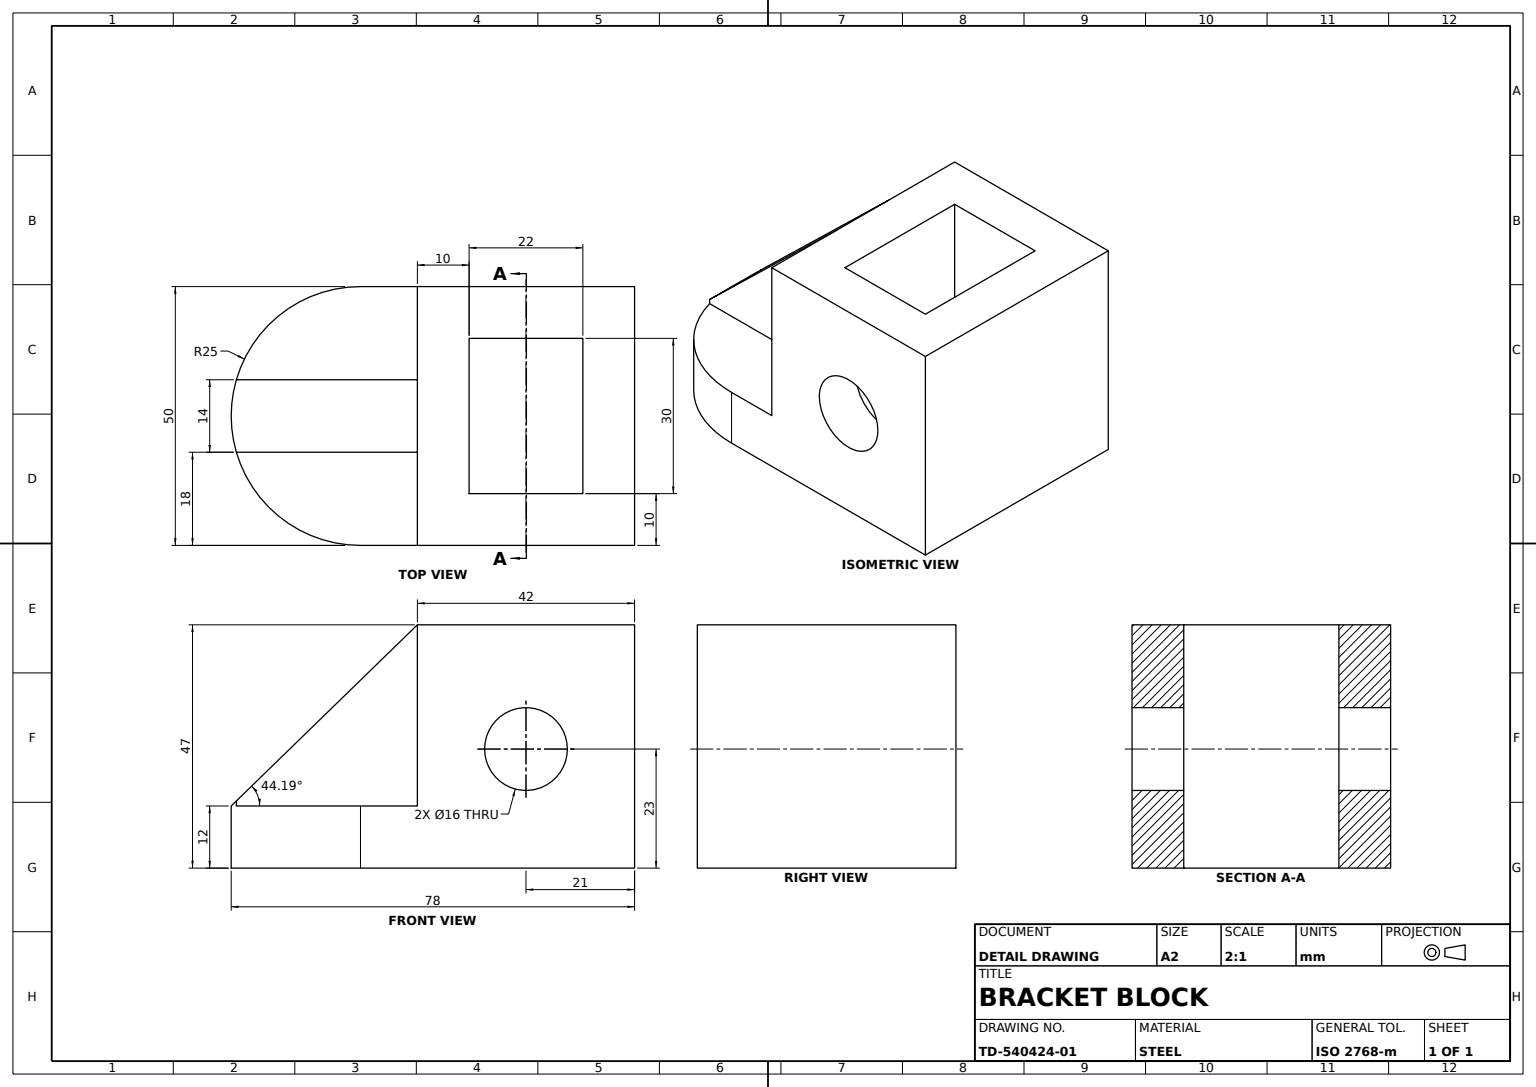
from build123d import *

# Parameters (mm, degrees)
BASE_PLATE_SKETCH_W      = 78
BASE_PLATE_SKETCH_H      = 12
BASE_PLATE_DEPTH         = 50
UPRIGHT_BLOCK_SKETCH_W   = 42
UPRIGHT_BLOCK_SKETCH_H   = 35
UPRIGHT_BLOCK_DEPTH      = 50
BLOCK_POCKET_SKETCH_W    = 30
BLOCK_POCKET_SKETCH_H    = 22
BLOCK_POCKET_30X22_DEPTH = 79.930349043
SIDE_CUT_1_SKETCH_R      = 8
SIDE_CUT_1_DEPTH         = 10
SIDE_START               = -10
SIDE_CUT_2_SKETCH_R      = 8
SIDE_CUT_2_DEPTH         = 10
GUSSET_RIB_14MM_REACH    = 63.863
GUSSET_RIB_SKETCH_WALL_W = 175.935063468
GUSSET_RIB_SKETCH_WALL_H = 14
FRONT_PROFILE_CUT_DEPTH  = 73.429275849
RIB_START                = -20
RIB_TRIM_CUT_DEPTH       = 20


with BuildPart() as part:
    # Base Plate Sketch → Base Plate (new body)
    with BuildSketch(Plane(origin=(0, 0, 0), x_dir=(0, 0, -1), z_dir=(1, 0, 0))):
        Rectangle(BASE_PLATE_SKETCH_W, BASE_PLATE_SKETCH_H)
    extrude(amount=-BASE_PLATE_DEPTH)

    # Upright Block Sketch → Upright Block (add)
    with BuildSketch(Plane(origin=(0, 0, 0), x_dir=(0, 0, -1), z_dir=(1, 0, 0))):
        with Locations((18, 23.5)):
            Rectangle(UPRIGHT_BLOCK_SKETCH_W, UPRIGHT_BLOCK_SKETCH_H)
    extrude(amount=-UPRIGHT_BLOCK_DEPTH)

    # Block Pocket Sketch → Block Pocket 30x22 (cut, through all)
    with BuildSketch(Plane(origin=(0, 41, 0), x_dir=(1, 0, 0), z_dir=(0, 1, 0))):
        with Locations((-25, 18)):
            Rectangle(BLOCK_POCKET_SKETCH_W, BLOCK_POCKET_SKETCH_H)
    extrude(amount=-BLOCK_POCKET_30X22_DEPTH, mode=Mode.SUBTRACT)

    # Side Cut 1 Sketch → Side Cut 1 (cut)
    with BuildSketch(Plane(origin=(0, 0, 0), x_dir=(0, 0, -1), z_dir=(1, 0, 0))):
        with Locations((18, 17)):
            Circle(SIDE_CUT_1_SKETCH_R)
    extrude(amount=-SIDE_CUT_1_DEPTH, mode=Mode.SUBTRACT)

    # Side Cut 2 Sketch → Side Cut 2 (cut)
    with BuildSketch(Plane.ZY.offset(50).offset(SIDE_START)):
        with Locations(Location((-18, 17, 0), (0, 0, 180))):
            Circle(SIDE_CUT_2_SKETCH_R)
    extrude(amount=SIDE_CUT_2_DEPTH, mode=Mode.SUBTRACT)

    # Gusset Rib Sketch wall → Gusset Rib 14mm (add, up to next)
    with BuildSketch(Plane(origin=(-25, 23.5, 21), x_dir=(0, 0.697078393292, -0.716994918814), z_dir=(0, 0.716994918814, 0.697078393292)), mode=Mode.PRIVATE) as gusset_rib_14mm_sk1:
        Rectangle(GUSSET_RIB_SKETCH_WALL_W, GUSSET_RIB_SKETCH_WALL_H)
    gusset_rib_14mm_tool1 = extrude(gusset_rib_14mm_sk1.sketch, amount=-GUSSET_RIB_14MM_REACH, mode=Mode.PRIVATE) - part.part
    add(gusset_rib_14mm_tool1.solids().sort_by_distance((-25, 23.5, 21))[0])

    # Front Profile Cut Sketch → Front Profile Cut (cut, through all)
    with BuildSketch(Plane(origin=(0, 6, 0), x_dir=(1, 0, 0), z_dir=(0, 1, 0))):
        with BuildLine():
            Line((-50, -39), (-25, -39))
            ThreePointArc((-25, -39), (-42.67766953, -31.67766953), (-50, -14))
            Line((-50, -14), (-50, -39))
        make_face()
        with BuildLine():
            Line((-18, -38), (-18, -39))
            Line((-18, -39), (0, -39))
            Line((0, -39), (0, -14))
            ThreePointArc((0, -14), (-5, -29), (-18, -38))
        make_face()
    extrude(amount=-FRONT_PROFILE_CUT_DEPTH, mode=Mode.SUBTRACT)

    # Rib Trim Cut Sketch → Rib Trim Cut (cut)
    with BuildSketch(Plane.XZ.offset(6).offset(RIB_START)):
        with BuildLine():
            Line((-25, 39), (-32, 39))
            Line((-32, 39), (-32, 38))
            ThreePointArc((-32, 38), (-28.535533906, 38.748737342), (-25, 39))
        make_face()
        with BuildLine():
            ThreePointArc((-18, 38), (-21.464466094, 38.748737342), (-25, 39))
            Line((-25, 39), (-18, 39))
            Line((-18, 39), (-18, 38))
        make_face()
    extrude(amount=RIB_TRIM_CUT_DEPTH, mode=Mode.SUBTRACT)


solid = part.part
